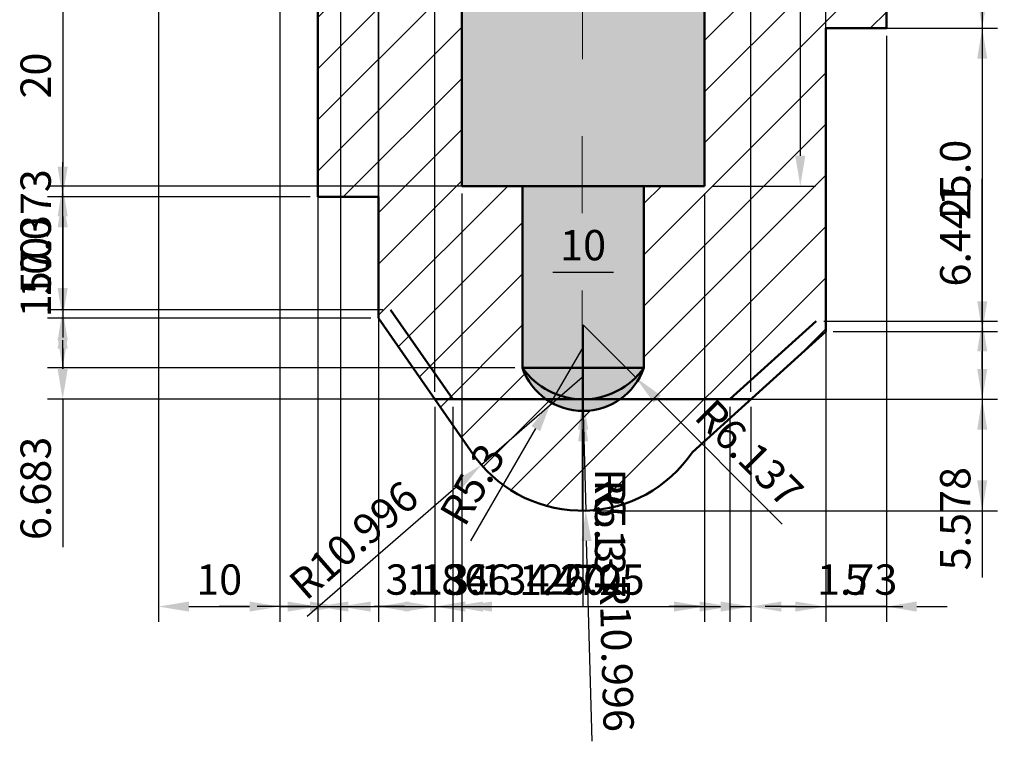
# Model space of a CAD drawing. Units: millimetres. Extents: x 1159 to 1466, y 1237 to 1440.
# Tile 4 of 6: x 1378 to 1459, y 1237 to 1296. Entities that reach past the tile are written whole.
import ezdxf

# ---------------------------------------------------------------- set-up
doc = ezdxf.new("R2010")
doc.units = ezdxf.units.MM
doc.linetypes.add('CENTER', pattern=[50.8, 31.75, -6.35, 6.35, -6.35])
for name, color, linetype, lineweight in [('M-CNTR', 1, 'CENTER', 18), ('M-DIMS', 2, 'Continuous', 25), ('M-HATC', 8, 'Continuous', 18), ('M-OUTL', 7, 'Continuous', 50)]:
    doc.layers.add(name, color=color, linetype=linetype, lineweight=lineweight)
doc.styles.get("Standard").update_dxf_attribs({"font": 'arial.ttf'})
doc.dimstyles.new('ISO-25', dxfattribs={"dimtxt": 2.5, "dimasz": 2.5, "dimexe": 1.25, "dimexo": 0.625, "dimtad": 1, "dimtxsty": 'Standard', "dimcen": 2.5, "dimadec": 0, "dimazin": 0, "dimtfac": 1, "dimtmove": 0, "dimatfit": 3, "dimfxl": 1, "dimarcsym": 0})

# ---------------------------------------------------------------- blocks, each defined once
blk = doc.blocks.new('*D42')
at = {"layer": 'Defpoints', "color": 0, "transparency": 16777216}
for p in [(1409.751, 1375.561), (1424.964, 1255.799), (1457.651, 1255.799)]:
    blk.add_point(p, dxfattribs=at)
at = {"layer": 'M-DIMS', "color": 0, "lineweight": -2, "transparency": 16777216}
for p, q in [((1410.376, 1375.561), (1458.901, 1375.561)), ((1457.651, 1373.061), (1457.651, 1258.299)), ((1425.589, 1255.799), (1458.901, 1255.799))]:
    blk.add_line(p, q, dxfattribs=at)
at = {"layer": 'M-DIMS', "color": 0, "transparency": 16777216}
for points in [[(1457.234, 1373.061), (1458.067, 1373.061), (1457.651, 1375.561)], [(1457.234, 1258.299), (1458.067, 1258.299), (1457.651, 1255.799)]]:
    blk.add_solid(points, dxfattribs=at)
at = {"layer": 'M-DIMS', "color": 0, "transparency": 16777216, "insert": (1455.749, 1315.68), "char_height": 2.5, "attachment_point": 5, "rotation": 90}
blk.add_mtext('119.76', dxfattribs=at)
blk = doc.blocks.new('*D44')
at = {"layer": 'Defpoints', "color": 0, "transparency": 16777216}
for p in [(1389.751, 1320.561), (1399.751, 1320.561), (1399.751, 1247.895)]:
    blk.add_point(p, dxfattribs=at)
at = {"layer": 'M-DIMS', "color": 0, "lineweight": -2, "transparency": 16777216}
for p, q in [((1389.751, 1319.936), (1389.751, 1246.645)), ((1399.751, 1319.936), (1399.751, 1246.645)), ((1392.251, 1247.895), (1397.251, 1247.895))]:
    blk.add_line(p, q, dxfattribs=at)
at = {"layer": 'M-DIMS', "color": 0, "transparency": 16777216}
for points in [[(1392.251, 1248.311), (1392.251, 1247.478), (1389.751, 1247.895)], [(1397.251, 1248.311), (1397.251, 1247.478), (1399.751, 1247.895)]]:
    blk.add_solid(points, dxfattribs=at)
at = {"layer": 'M-DIMS', "color": 0, "transparency": 16777216, "insert": (1394.751, 1249.796), "char_height": 2.5, "attachment_point": 5}
blk.add_mtext('10', dxfattribs=at)
blk = doc.blocks.new('*D46')
at = {"layer": 'Defpoints', "color": 0, "transparency": 16777216}
for p in [(1414.751, 1282.561), (1434.751, 1282.561), (1434.751, 1247.895)]:
    blk.add_point(p, dxfattribs=at)
at = {"layer": 'M-DIMS', "color": 0, "lineweight": -2, "transparency": 16777216}
for p, q in [((1414.751, 1281.936), (1414.751, 1246.645)), ((1434.751, 1281.936), (1434.751, 1246.645)), ((1417.251, 1247.895), (1432.251, 1247.895))]:
    blk.add_line(p, q, dxfattribs=at)
at = {"layer": 'M-DIMS', "color": 0, "transparency": 16777216}
for points in [[(1417.251, 1248.311), (1417.251, 1247.478), (1414.751, 1247.895)], [(1432.251, 1248.311), (1432.251, 1247.478), (1434.751, 1247.895)]]:
    blk.add_solid(points, dxfattribs=at)
at = {"layer": 'M-DIMS', "color": 0, "transparency": 16777216, "insert": (1424.751, 1249.796), "char_height": 2.5, "attachment_point": 5}
blk.add_mtext('20', dxfattribs=at)
blk = doc.blocks.new('*D47')
at = {"layer": 'Defpoints', "color": 0, "transparency": 16777216}
for p in [(1434.751, 1317.561), (1434.751, 1282.561), (1442.651, 1282.561)]:
    blk.add_point(p, dxfattribs=at)
at = {"layer": 'M-DIMS', "color": 0, "lineweight": -2, "transparency": 16777216}
for p, q in [((1435.376, 1317.561), (1443.901, 1317.561)), ((1442.651, 1315.061), (1442.651, 1285.061)), ((1435.376, 1282.561), (1443.901, 1282.561))]:
    blk.add_line(p, q, dxfattribs=at)
at = {"layer": 'M-DIMS', "color": 0, "transparency": 16777216}
for points in [[(1442.234, 1315.061), (1443.067, 1315.061), (1442.651, 1317.561)], [(1442.234, 1285.061), (1443.067, 1285.061), (1442.651, 1282.561)]]:
    blk.add_solid(points, dxfattribs=at)
at = {"layer": 'M-DIMS', "color": 0, "transparency": 16777216, "insert": (1440.749, 1300.061), "char_height": 2.5, "attachment_point": 5, "rotation": 90}
blk.add_mtext('35', dxfattribs=at)
blk = doc.blocks.new('*D48')
at = {"layer": 'Defpoints', "color": 0, "transparency": 16777216}
for p in [(1429.751, 1275.461), (1419.751, 1267.561), (1429.751, 1267.561)]:
    blk.add_point(p, dxfattribs=at)
at = {"layer": 'M-DIMS', "color": 0, "lineweight": -2, "transparency": 16777216}
for p, q in [((1419.751, 1268.186), (1419.751, 1276.711)), ((1429.751, 1268.186), (1429.751, 1276.711)), ((1422.251, 1275.461), (1427.251, 1275.461))]:
    blk.add_line(p, q, dxfattribs=at)
at = {"layer": 'M-DIMS', "color": 0, "transparency": 16777216}
for points in [[(1422.251, 1275.878), (1422.251, 1275.044), (1419.751, 1275.461)], [(1427.251, 1275.878), (1427.251, 1275.044), (1429.751, 1275.461)]]:
    blk.add_solid(points, dxfattribs=at)
at = {"layer": 'M-DIMS', "color": 0, "transparency": 16777216, "insert": (1424.751, 1277.362), "char_height": 2.5, "attachment_point": 5}
blk.add_mtext('10', dxfattribs=at)
blk = doc.blocks.new('*D49')
at = {"layer": 'Defpoints', "color": 0, "transparency": 16777216}
for p in [(1444.751, 1295.561), (1449.751, 1295.561), (1444.751, 1247.895)]:
    blk.add_point(p, dxfattribs=at)
at = {"layer": 'M-DIMS', "color": 0, "lineweight": -2, "transparency": 16777216}
for p, q in [((1444.751, 1294.936), (1444.751, 1246.645)), ((1449.751, 1294.936), (1449.751, 1246.645)), ((1442.251, 1247.895), (1439.751, 1247.895)), ((1449.751, 1247.895), (1444.751, 1247.895)), ((1452.251, 1247.895), (1454.751, 1247.895))]:
    blk.add_line(p, q, dxfattribs=at)
at = {"layer": 'M-DIMS', "color": 0, "transparency": 16777216}
for points in [[(1442.251, 1248.311), (1442.251, 1247.478), (1444.751, 1247.895)], [(1452.251, 1248.311), (1452.251, 1247.478), (1449.751, 1247.895)]]:
    blk.add_solid(points, dxfattribs=at)
at = {"layer": 'M-DIMS', "color": 0, "transparency": 16777216, "insert": (1447.251, 1249.791), "char_height": 2.5, "attachment_point": 5}
blk.add_mtext('5', dxfattribs=at)
blk = doc.blocks.new('*D50')
at = {"layer": 'Defpoints', "color": 0, "transparency": 16777216}
for p in [(1449.751, 1315.561), (1449.751, 1295.561), (1457.651, 1295.561)]:
    blk.add_point(p, dxfattribs=at)
at = {"layer": 'M-DIMS', "color": 0, "lineweight": -2, "transparency": 16777216}
for p, q in [((1450.376, 1315.561), (1458.901, 1315.561)), ((1457.651, 1313.061), (1457.651, 1298.061)), ((1450.376, 1295.561), (1458.901, 1295.561))]:
    blk.add_line(p, q, dxfattribs=at)
at = {"layer": 'M-DIMS', "color": 0, "transparency": 16777216}
for points in [[(1457.234, 1313.061), (1458.067, 1313.061), (1457.651, 1315.561)], [(1457.234, 1298.061), (1458.067, 1298.061), (1457.651, 1295.561)]]:
    blk.add_solid(points, dxfattribs=at)
at = {"layer": 'M-DIMS', "color": 0, "transparency": 16777216, "insert": (1455.749, 1305.561), "char_height": 2.5, "attachment_point": 5, "rotation": 90}
blk.add_mtext('20', dxfattribs=at)
blk = doc.blocks.new('*D51')
at = {"layer": 'Defpoints', "color": 0, "transparency": 16777216}
for p in [(1402.885, 1301.665), (1381.851, 1281.665), (1402.885, 1281.665)]:
    blk.add_point(p, dxfattribs=at)
at = {"layer": 'M-DIMS', "color": 0, "lineweight": -2, "transparency": 16777216}
for p, q in [((1402.26, 1301.665), (1380.601, 1301.665)), ((1381.851, 1299.165), (1381.851, 1284.165)), ((1402.26, 1281.665), (1380.601, 1281.665))]:
    blk.add_line(p, q, dxfattribs=at)
at = {"layer": 'M-DIMS', "color": 0, "transparency": 16777216}
for points in [[(1381.434, 1299.165), (1382.267, 1299.165), (1381.851, 1301.665)], [(1381.434, 1284.165), (1382.267, 1284.165), (1381.851, 1281.665)]]:
    blk.add_solid(points, dxfattribs=at)
at = {"layer": 'M-DIMS', "color": 0, "transparency": 16777216, "insert": (1379.949, 1291.665), "char_height": 2.5, "attachment_point": 5, "rotation": 90}
blk.add_mtext('20', dxfattribs=at)
blk = doc.blocks.new('*D54')
at = {"layer": 'Defpoints', "color": 0, "transparency": 16777216}
for p in [(1424.659, 1266.79), (1424.964, 1255.799)]:
    blk.add_point(p, dxfattribs=at)
at = {"layer": 'M-DIMS', "color": 0, "lineweight": -2, "transparency": 16777216}
for p, q in [((1424.659, 1266.79), (1424.964, 1255.799)), ((1425.492, 1236.787), (1425.033, 1253.3))]:
    blk.add_line(p, q, dxfattribs=at)
at = {"layer": 'M-DIMS', "color": 0, "transparency": 16777216}
blk.add_solid([(1425.45, 1253.311), (1424.617, 1253.288), (1424.964, 1255.799)], dxfattribs=at)
at = {"layer": 'M-DIMS', "color": 0, "transparency": 16777216, "insert": (1427.198, 1243.846), "char_height": 2.5, "attachment_point": 5, "rotation": 271.59062}
blk.add_mtext('R10.996', dxfattribs=at)
blk = doc.blocks.new('*D55')
at = {"layer": 'Defpoints', "color": 0, "transparency": 16777216}
for p in [(1424.751, 1271.12), (1424.751, 1264.983)]:
    blk.add_point(p, dxfattribs=at)
at = {"layer": 'M-DIMS', "color": 0, "lineweight": -2, "transparency": 16777216}
for p, q in [((1424.751, 1271.12), (1424.751, 1264.983)), ((1424.752, 1247.904), (1424.751, 1262.483))]:
    blk.add_line(p, q, dxfattribs=at)
at = {"layer": 'M-DIMS', "color": 0, "transparency": 16777216}
blk.add_solid([(1425.168, 1262.483), (1424.334, 1262.483), (1424.751, 1264.983)], dxfattribs=at)
at = {"layer": 'M-DIMS', "color": 0, "transparency": 16777216, "insert": (1426.654, 1253.943), "char_height": 2.5, "attachment_point": 5, "rotation": 270.0019}
blk.add_mtext('R6.137', dxfattribs=at)
blk = doc.blocks.new('*D56')
at = {"layer": 'Defpoints', "color": 0, "transparency": 16777216}
for p in [(1424.751, 1269.318), (1424.751, 1264.018)]:
    blk.add_point(p, dxfattribs=at)
at = {"layer": 'M-DIMS', "color": 0, "lineweight": -2, "transparency": 16777216}
for p, q in [((1424.751, 1269.318), (1424.751, 1264.018)), ((1424.752, 1250.824), (1424.751, 1261.518))]:
    blk.add_line(p, q, dxfattribs=at)
at = {"layer": 'M-DIMS', "color": 0, "transparency": 16777216}
blk.add_solid([(1425.168, 1261.518), (1424.334, 1261.518), (1424.751, 1264.018)], dxfattribs=at)
at = {"layer": 'M-DIMS', "color": 0, "transparency": 16777216, "insert": (1426.654, 1254.921), "char_height": 2.5, "attachment_point": 5, "rotation": 270.00221}
blk.add_mtext('R5.3', dxfattribs=at)
blk = doc.blocks.new('*D61')
at = {"layer": 'Defpoints', "color": 0, "transparency": 16777216}
for p in [(1444.751, 1295.561), (1444.751, 1270.561), (1457.651, 1270.561)]:
    blk.add_point(p, dxfattribs=at)
at = {"layer": 'M-DIMS', "color": 0, "lineweight": -2, "transparency": 16777216}
for p, q in [((1445.376, 1295.561), (1458.901, 1295.561)), ((1457.651, 1293.061), (1457.651, 1273.061)), ((1445.376, 1270.561), (1458.901, 1270.561))]:
    blk.add_line(p, q, dxfattribs=at)
at = {"layer": 'M-DIMS', "color": 0, "transparency": 16777216}
for points in [[(1457.234, 1293.061), (1458.067, 1293.061), (1457.651, 1295.561)], [(1457.234, 1273.061), (1458.067, 1273.061), (1457.651, 1270.561)]]:
    blk.add_solid(points, dxfattribs=at)
at = {"layer": 'M-DIMS', "color": 0, "transparency": 16777216, "insert": (1455.749, 1283.061), "char_height": 2.5, "attachment_point": 5, "rotation": 90}
blk.add_mtext('25.0', dxfattribs=at)
blk = doc.blocks.new('*D65')
at = {"layer": 'Defpoints', "color": 0, "transparency": 16777216}
for p in [(1399.751, 1315.561), (1402.885, 1301.665), (1402.885, 1247.895)]:
    blk.add_point(p, dxfattribs=at)
at = {"layer": 'M-DIMS', "color": 0, "lineweight": -2, "transparency": 16777216}
for p, q in [((1399.751, 1314.936), (1399.751, 1246.645)), ((1402.885, 1301.04), (1402.885, 1246.645)), ((1397.251, 1247.895), (1394.751, 1247.895)), ((1399.751, 1247.895), (1402.885, 1247.895)), ((1405.385, 1247.895), (1417.559, 1247.895))]:
    blk.add_line(p, q, dxfattribs=at)
at = {"layer": 'M-DIMS', "color": 0, "transparency": 16777216}
for points in [[(1397.251, 1248.311), (1397.251, 1247.478), (1399.751, 1247.895)], [(1405.385, 1248.311), (1405.385, 1247.478), (1402.885, 1247.895)]]:
    blk.add_solid(points, dxfattribs=at)
at = {"layer": 'M-DIMS', "color": 0, "transparency": 16777216, "insert": (1412.722, 1249.797), "char_height": 2.5, "attachment_point": 5}
blk.add_mtext('3.134', dxfattribs=at)
blk = doc.blocks.new('*D66')
at = {"layer": 'Defpoints', "color": 0, "transparency": 16777216}
for p in [(1404.751, 1315.561), (1402.885, 1301.665), (1404.751, 1247.895)]:
    blk.add_point(p, dxfattribs=at)
at = {"layer": 'M-DIMS', "color": 0, "lineweight": -2, "transparency": 16777216}
for p, q in [((1404.751, 1314.936), (1404.751, 1246.645)), ((1402.885, 1301.04), (1402.885, 1246.645)), ((1400.385, 1247.895), (1397.885, 1247.895)), ((1402.885, 1247.895), (1404.751, 1247.895)), ((1407.251, 1247.895), (1419.2, 1247.895))]:
    blk.add_line(p, q, dxfattribs=at)
at = {"layer": 'M-DIMS', "color": 0, "transparency": 16777216}
for points in [[(1400.385, 1248.311), (1400.385, 1247.478), (1402.885, 1247.895)], [(1407.251, 1248.311), (1407.251, 1247.478), (1404.751, 1247.895)]]:
    blk.add_solid(points, dxfattribs=at)
at = {"layer": 'M-DIMS', "color": 0, "transparency": 16777216, "insert": (1414.475, 1249.796), "char_height": 2.5, "attachment_point": 5}
blk.add_mtext('1.866', dxfattribs=at)
blk = doc.blocks.new('*D67')
at = {"layer": 'Defpoints', "color": 0, "transparency": 16777216}
for p in [(1404.751, 1315.561), (1407.885, 1311.665), (1407.885, 1247.895)]:
    blk.add_point(p, dxfattribs=at)
at = {"layer": 'M-DIMS', "color": 0, "lineweight": -2, "transparency": 16777216}
for p, q in [((1404.751, 1314.936), (1404.751, 1246.645)), ((1407.885, 1311.04), (1407.885, 1246.645)), ((1402.251, 1247.895), (1399.751, 1247.895)), ((1404.751, 1247.895), (1407.885, 1247.895)), ((1410.385, 1247.895), (1422.559, 1247.895))]:
    blk.add_line(p, q, dxfattribs=at)
at = {"layer": 'M-DIMS', "color": 0, "transparency": 16777216}
for points in [[(1402.251, 1248.311), (1402.251, 1247.478), (1404.751, 1247.895)], [(1410.385, 1248.311), (1410.385, 1247.478), (1407.885, 1247.895)]]:
    blk.add_solid(points, dxfattribs=at)
at = {"layer": 'M-DIMS', "color": 0, "transparency": 16777216, "insert": (1417.722, 1249.797), "char_height": 2.5, "attachment_point": 5}
blk.add_mtext('3.134', dxfattribs=at)
blk = doc.blocks.new('*D68')
at = {"layer": 'Defpoints', "color": 0, "transparency": 16777216}
for p in [(1402.885, 1281.665), (1381.851, 1271.665), (1407.885, 1271.665)]:
    blk.add_point(p, dxfattribs=at)
at = {"layer": 'M-DIMS', "color": 0, "lineweight": -2, "transparency": 16777216}
for p, q in [((1402.26, 1281.665), (1380.601, 1281.665)), ((1381.851, 1279.165), (1381.851, 1274.165)), ((1407.26, 1271.665), (1380.601, 1271.665))]:
    blk.add_line(p, q, dxfattribs=at)
at = {"layer": 'M-DIMS', "color": 0, "transparency": 16777216}
for points in [[(1381.434, 1279.165), (1382.267, 1279.165), (1381.851, 1281.665)], [(1381.434, 1274.165), (1382.267, 1274.165), (1381.851, 1271.665)]]:
    blk.add_solid(points, dxfattribs=at)
at = {"layer": 'M-DIMS', "color": 0, "transparency": 16777216, "insert": (1379.949, 1276.665), "char_height": 2.5, "attachment_point": 5, "rotation": 90}
blk.add_mtext('10.0', dxfattribs=at)
blk = doc.blocks.new('*D69')
at = {"layer": 'Defpoints', "color": 0, "transparency": 16777216}
for p in [(1407.885, 1271.665), (1381.851, 1264.983), (1412.534, 1264.983)]:
    blk.add_point(p, dxfattribs=at)
at = {"layer": 'M-DIMS', "color": 0, "lineweight": -2, "transparency": 16777216}
for p, q in [((1407.26, 1271.665), (1380.601, 1271.665)), ((1381.851, 1269.165), (1381.851, 1267.483)), ((1411.909, 1264.983), (1380.601, 1264.983)), ((1381.851, 1264.983), (1381.851, 1252.783))]:
    blk.add_line(p, q, dxfattribs=at)
at = {"layer": 'M-DIMS', "color": 0, "transparency": 16777216}
for points in [[(1381.434, 1269.165), (1382.267, 1269.165), (1381.851, 1271.665)], [(1381.434, 1267.483), (1382.267, 1267.483), (1381.851, 1264.983)]]:
    blk.add_solid(points, dxfattribs=at)
at = {"layer": 'M-DIMS', "color": 0, "transparency": 16777216, "insert": (1379.949, 1257.633), "char_height": 2.5, "attachment_point": 5, "rotation": 90}
blk.add_mtext('6.683', dxfattribs=at)
blk = doc.blocks.new('*D70')
at = {"layer": 'Defpoints', "color": 0, "transparency": 16777216}
for p in [(1444.751, 1270.561), (1438.586, 1264.983), (1457.651, 1264.983)]:
    blk.add_point(p, dxfattribs=at)
at = {"layer": 'M-DIMS', "color": 0, "lineweight": -2, "transparency": 16777216}
for p, q in [((1457.651, 1273.061), (1457.651, 1275.561)), ((1445.376, 1270.561), (1458.901, 1270.561)), ((1457.651, 1270.561), (1457.651, 1264.983)), ((1439.211, 1264.983), (1458.901, 1264.983)), ((1457.651, 1262.483), (1457.651, 1250.291))]:
    blk.add_line(p, q, dxfattribs=at)
at = {"layer": 'M-DIMS', "color": 0, "transparency": 16777216}
for points in [[(1457.234, 1273.061), (1458.067, 1273.061), (1457.651, 1270.561)], [(1457.234, 1262.483), (1458.067, 1262.483), (1457.651, 1264.983)]]:
    blk.add_solid(points, dxfattribs=at)
at = {"layer": 'M-DIMS', "color": 0, "transparency": 16777216, "insert": (1455.749, 1255.137), "char_height": 2.5, "attachment_point": 5, "rotation": 90}
blk.add_mtext('5.578', dxfattribs=at)
blk = doc.blocks.new('*D71')
at = {"layer": 'Defpoints', "color": 0, "transparency": 16777216}
for p in [(1443.97, 1271.424), (1457.651, 1271.424), (1436.851, 1264.983)]:
    blk.add_point(p, dxfattribs=at)
at = {"layer": 'M-DIMS', "color": 0, "lineweight": -2, "transparency": 16777216}
for p, q in [((1457.651, 1271.424), (1457.651, 1283.141)), ((1444.595, 1271.424), (1458.901, 1271.424)), ((1457.651, 1267.483), (1457.651, 1268.924)), ((1437.476, 1264.983), (1458.901, 1264.983))]:
    blk.add_line(p, q, dxfattribs=at)
at = {"layer": 'M-DIMS', "color": 0, "transparency": 16777216}
for points in [[(1457.234, 1268.924), (1458.067, 1268.924), (1457.651, 1271.424)], [(1457.234, 1267.483), (1458.067, 1267.483), (1457.651, 1264.983)]]:
    blk.add_solid(points, dxfattribs=at)
at = {"layer": 'M-DIMS', "color": 0, "transparency": 16777216, "insert": (1455.749, 1278.533), "char_height": 2.5, "attachment_point": 5, "rotation": 90}
blk.add_mtext('6.441', dxfattribs=at)
blk = doc.blocks.new('*D72')
at = {"layer": 'Defpoints', "color": 0, "transparency": 16777216}
for p in [(1381.851, 1272.355), (1408.877, 1272.355), (1414.006, 1264.983)]:
    blk.add_point(p, dxfattribs=at)
at = {"layer": 'M-DIMS', "color": 0, "lineweight": -2, "transparency": 16777216}
for p, q in [((1381.851, 1272.355), (1381.851, 1284.521)), ((1408.252, 1272.355), (1380.601, 1272.355)), ((1381.851, 1267.483), (1381.851, 1269.855)), ((1413.381, 1264.983), (1380.601, 1264.983))]:
    blk.add_line(p, q, dxfattribs=at)
at = {"layer": 'M-DIMS', "color": 0, "transparency": 16777216}
for points in [[(1381.434, 1269.855), (1382.267, 1269.855), (1381.851, 1272.355)], [(1381.434, 1267.483), (1382.267, 1267.483), (1381.851, 1264.983)]]:
    blk.add_solid(points, dxfattribs=at)
at = {"layer": 'M-DIMS', "color": 0, "transparency": 16777216, "insert": (1379.949, 1279.688), "char_height": 2.5, "attachment_point": 5, "rotation": 90}
blk.add_mtext('7.373', dxfattribs=at)
blk = doc.blocks.new('*D73')
at = {"layer": 'Defpoints', "color": 0, "transparency": 16777216}
for p in [(1412.534, 1264.983), (1438.586, 1264.983), (1438.586, 1247.895)]:
    blk.add_point(p, dxfattribs=at)
at = {"layer": 'M-DIMS', "color": 0, "lineweight": -2, "transparency": 16777216}
for p, q in [((1412.534, 1264.358), (1412.534, 1246.645)), ((1438.586, 1264.358), (1438.586, 1246.645)), ((1415.034, 1247.895), (1436.086, 1247.895))]:
    blk.add_line(p, q, dxfattribs=at)
at = {"layer": 'M-DIMS', "color": 0, "transparency": 16777216}
for points in [[(1415.034, 1248.311), (1415.034, 1247.478), (1412.534, 1247.895)], [(1436.086, 1248.311), (1436.086, 1247.478), (1438.586, 1247.895)]]:
    blk.add_solid(points, dxfattribs=at)
at = {"layer": 'M-DIMS', "color": 0, "transparency": 16777216, "insert": (1425.56, 1249.796), "char_height": 2.5, "attachment_point": 5}
blk.add_mtext('26.05', dxfattribs=at)
blk = doc.blocks.new('*D74')
at = {"layer": 'Defpoints', "color": 0, "transparency": 16777216}
for p in [(1412.534, 1383.461), (1407.885, 1271.665), (1412.534, 1264.983)]:
    blk.add_point(p, dxfattribs=at)
at = {"layer": 'M-DIMS', "color": 0, "lineweight": -2, "transparency": 16777216}
for p, q in [((1407.885, 1272.29), (1407.885, 1384.711)), ((1412.534, 1265.608), (1412.534, 1384.711)), ((1405.385, 1383.461), (1402.885, 1383.461)), ((1407.885, 1383.461), (1412.534, 1383.461)), ((1415.034, 1383.461), (1427.326, 1383.461))]:
    blk.add_line(p, q, dxfattribs=at)
at = {"layer": 'M-DIMS', "color": 0, "transparency": 16777216}
for points in [[(1405.385, 1383.878), (1405.385, 1383.044), (1407.885, 1383.461)], [(1415.034, 1383.878), (1415.034, 1383.044), (1412.534, 1383.461)]]:
    blk.add_solid(points, dxfattribs=at)
at = {"layer": 'M-DIMS', "color": 0, "transparency": 16777216, "insert": (1422.43, 1385.362), "char_height": 2.5, "attachment_point": 5}
blk.add_mtext('4.649', dxfattribs=at)
blk = doc.blocks.new('*D75')
at = {"layer": 'Defpoints', "color": 0, "transparency": 16777216}
for p in [(1444.751, 1383.461), (1444.751, 1270.561), (1438.586, 1264.983)]:
    blk.add_point(p, dxfattribs=at)
at = {"layer": 'M-DIMS', "color": 0, "lineweight": -2, "transparency": 16777216}
for p, q in [((1438.586, 1265.608), (1438.586, 1384.711)), ((1444.751, 1271.186), (1444.751, 1384.711)), ((1436.086, 1383.461), (1433.586, 1383.461)), ((1438.586, 1383.461), (1444.751, 1383.461)), ((1447.251, 1383.461), (1459.469, 1383.461))]:
    blk.add_line(p, q, dxfattribs=at)
at = {"layer": 'M-DIMS', "color": 0, "transparency": 16777216}
for points in [[(1436.086, 1383.878), (1436.086, 1383.044), (1438.586, 1383.461)], [(1447.251, 1383.878), (1447.251, 1383.044), (1444.751, 1383.461)]]:
    blk.add_solid(points, dxfattribs=at)
at = {"layer": 'M-DIMS', "color": 0, "transparency": 16777216, "insert": (1454.61, 1385.362), "char_height": 2.5, "attachment_point": 5}
blk.add_mtext('6.165', dxfattribs=at)
blk = doc.blocks.new('*D76')
at = {"layer": 'Defpoints', "color": 0, "transparency": 16777216}
for p in [(1412.534, 1264.983), (1414.006, 1264.983), (1414.006, 1247.895)]:
    blk.add_point(p, dxfattribs=at)
at = {"layer": 'M-DIMS', "color": 0, "lineweight": -2, "transparency": 16777216}
for p, q in [((1412.534, 1264.358), (1412.534, 1246.645)), ((1414.006, 1264.358), (1414.006, 1246.645)), ((1410.034, 1247.895), (1407.534, 1247.895)), ((1412.534, 1247.895), (1414.006, 1247.895)), ((1416.506, 1247.895), (1428.432, 1247.895))]:
    blk.add_line(p, q, dxfattribs=at)
at = {"layer": 'M-DIMS', "color": 0, "transparency": 16777216}
for points in [[(1410.034, 1248.311), (1410.034, 1247.478), (1412.534, 1247.895)], [(1416.506, 1248.311), (1416.506, 1247.478), (1414.006, 1247.895)]]:
    blk.add_solid(points, dxfattribs=at)
at = {"layer": 'M-DIMS', "color": 0, "transparency": 16777216, "insert": (1423.719, 1249.775), "char_height": 2.5, "attachment_point": 5}
blk.add_mtext('1.472', dxfattribs=at)
blk = doc.blocks.new('*D77')
at = {"layer": 'Defpoints', "color": 0, "transparency": 16777216}
for p in [(1436.851, 1264.983), (1438.586, 1264.983), (1438.586, 1247.895)]:
    blk.add_point(p, dxfattribs=at)
at = {"layer": 'M-DIMS', "color": 0, "lineweight": -2, "transparency": 16777216}
for p, q in [((1436.851, 1264.358), (1436.851, 1246.645)), ((1438.586, 1264.358), (1438.586, 1246.645)), ((1434.351, 1247.895), (1431.851, 1247.895)), ((1436.851, 1247.895), (1438.586, 1247.895)), ((1441.086, 1247.895), (1451.094, 1247.895))]:
    blk.add_line(p, q, dxfattribs=at)
at = {"layer": 'M-DIMS', "color": 0, "transparency": 16777216}
for points in [[(1434.351, 1248.311), (1434.351, 1247.478), (1436.851, 1247.895)], [(1441.086, 1248.311), (1441.086, 1247.478), (1438.586, 1247.895)]]:
    blk.add_solid(points, dxfattribs=at)
at = {"layer": 'M-DIMS', "color": 0, "transparency": 16777216, "insert": (1447.34, 1249.797), "char_height": 2.5, "attachment_point": 5}
blk.add_mtext('1.73', dxfattribs=at)
blk = doc.blocks.new('*D78')
at = {"layer": 'Defpoints', "color": 0, "transparency": 16777216}
for p in [(1419.751, 1282.561), (1381.851, 1267.561), (1419.751, 1267.561)]:
    blk.add_point(p, dxfattribs=at)
at = {"layer": 'M-DIMS', "color": 0, "lineweight": -2, "transparency": 16777216}
for p, q in [((1419.126, 1282.561), (1380.601, 1282.561)), ((1381.851, 1280.061), (1381.851, 1270.061)), ((1419.126, 1267.561), (1380.601, 1267.561))]:
    blk.add_line(p, q, dxfattribs=at)
at = {"layer": 'M-DIMS', "color": 0, "transparency": 16777216}
for points in [[(1381.434, 1280.061), (1382.267, 1280.061), (1381.851, 1282.561)], [(1381.434, 1270.061), (1382.267, 1270.061), (1381.851, 1267.561)]]:
    blk.add_solid(points, dxfattribs=at)
at = {"layer": 'M-DIMS', "color": 0, "transparency": 16777216, "insert": (1379.949, 1275.061), "char_height": 2.5, "attachment_point": 5, "rotation": 90}
blk.add_mtext('15.0', dxfattribs=at)
blk = doc.blocks.new('*D88')
at = {"layer": 'Defpoints', "color": 0, "transparency": 16777216}
for p in [(1424.659, 1266.79), (1416.362, 1259.575)]:
    blk.add_point(p, dxfattribs=at)
at = {"layer": 'M-DIMS', "color": 0, "lineweight": -2, "transparency": 16777216}
for p, q in [((1424.659, 1266.79), (1416.362, 1259.575)), ((1402.01, 1247.094), (1414.475, 1257.934))]:
    blk.add_line(p, q, dxfattribs=at)
at = {"layer": 'M-DIMS', "color": 0, "transparency": 16777216}
blk.add_solid([(1414.202, 1258.249), (1414.749, 1257.62), (1416.362, 1259.575)], dxfattribs=at)
at = {"layer": 'M-DIMS', "color": 0, "transparency": 16777216, "insert": (1406.052, 1253.129), "char_height": 2.5, "attachment_point": 5, "rotation": 41.01102}
blk.add_mtext('R10.996', dxfattribs=at)
blk = doc.blocks.new('*D89')
at = {"layer": 'Defpoints', "color": 0, "transparency": 16777216}
for p in [(1424.751, 1271.12), (1429.085, 1266.775)]:
    blk.add_point(p, dxfattribs=at)
at = {"layer": 'M-DIMS', "color": 0, "lineweight": -2, "transparency": 16777216}
for p, q in [((1424.751, 1271.12), (1429.085, 1266.775)), ((1441.147, 1254.683), (1430.851, 1265.005))]:
    blk.add_line(p, q, dxfattribs=at)
at = {"layer": 'M-DIMS', "color": 0, "transparency": 16777216}
blk.add_solid([(1431.146, 1265.299), (1430.556, 1264.711), (1429.085, 1266.775)], dxfattribs=at)
at = {"layer": 'M-DIMS', "color": 0, "transparency": 16777216, "insert": (1438.228, 1260.303), "char_height": 2.5, "attachment_point": 5, "rotation": 314.92911}
blk.add_mtext('R6.137', dxfattribs=at)
blk = doc.blocks.new('*D90')
at = {"layer": 'Defpoints', "color": 0, "transparency": 16777216}
for p in [(1424.751, 1269.318), (1422.1, 1264.729)]:
    blk.add_point(p, dxfattribs=at)
at = {"layer": 'M-DIMS', "color": 0, "lineweight": -2, "transparency": 16777216}
for p, q in [((1424.751, 1269.318), (1422.1, 1264.729)), ((1415.499, 1253.305), (1420.849, 1262.565))]:
    blk.add_line(p, q, dxfattribs=at)
at = {"layer": 'M-DIMS', "color": 0, "transparency": 16777216}
blk.add_solid([(1420.488, 1262.773), (1421.21, 1262.356), (1422.1, 1264.729)], dxfattribs=at)
at = {"layer": 'M-DIMS', "color": 0, "transparency": 16777216, "insert": (1415.902, 1257.804), "char_height": 2.5, "attachment_point": 5, "rotation": 59.98324}
blk.add_mtext('R5.3', dxfattribs=at)

msp = doc.modelspace()

# ---------------------------------------------------------------- hatches: boundary and pattern name
at = {"layer": 'M-HATC'}
h = msp.add_hatch(dxfattribs=at)
h.set_pattern_fill('ANSI31', color=256, scale=0.94)
h.set_pattern_definition([(45, (0, -76.8912), (-2.11036, 2.11036), [])])
h.paths.add_polyline_path([(1414.6374, 1375.561), (1409.7508, 1375.561), (1409.7508, 1335.561), (1414.6374, 1335.561)])
h.paths.add_polyline_path([(1439.7508, 1375.561), (1434.4515, 1375.561), (1434.4515, 1335.561), (1439.7508, 1335.561)])
h.paths.add_polyline_path([(1449.7508, 1315.561), (1444.7508, 1315.561), (1444.7508, 1320.561), (1449.7508, 1320.561), (1449.7508, 1335.561), (1439.7508, 1335.561), (1439.7508, 1320.561), (1429.7508, 1320.561), (1429.7508, 1317.561), (1434.7508, 1317.561), (1434.7508, 1282.561), (1429.7508, 1282.561), (1429.7508, 1267.561, -0.1562704), (1427.7989, 1264.9827), (1438.5857, 1264.9827), (1444.7508, 1270.561), (1444.7508, 1275.561), (1444.7508, 1295.561), (1449.7508, 1295.561)])
h.paths.add_polyline_path([(1414.7508, 1317.561), (1419.7508, 1317.561), (1419.7508, 1320.561), (1409.7508, 1320.561), (1409.7508, 1335.561), (1399.7508, 1335.561), (1399.7508, 1330.561), (1389.7508, 1330.561), (1389.7508, 1320.561), (1399.7508, 1320.561), (1399.7508, 1315.561), (1404.7508, 1315.561), (1407.8849, 1311.6652), (1407.8849, 1301.6652), (1402.8849, 1301.6652), (1402.8849, 1281.6652), (1407.8849, 1281.6652), (1407.8849, 1271.6652), (1412.5343, 1264.9827), (1421.7027, 1264.9827, -0.1562704), (1419.7508, 1267.561), (1419.7508, 1282.561), (1414.7508, 1282.561)])
h.paths.add_polyline_path([(1424.6651, 1264.0191, -0.1502665), (1421.7027, 1264.9827), (1412.5343, 1264.9827), (1415.9205, 1260.1158, 0.2337513), (1424.6588, 1255.7945)])
h.paths.add_polyline_path([(1433.7538, 1260.6108), (1438.5857, 1264.9827), (1427.7989, 1264.9827, -0.1585441), (1424.6651, 1264.0191), (1424.6588, 1255.7945, 0.248431)])
h = msp.add_hatch(color=256, dxfattribs=at)
h.set_gradient(color1=(34, 52, 110), color2=(0, 0, 0))
h.paths.add_polyline_path([(1424.7508, 1375.561), (1414.6374, 1375.561), (1414.6374, 1335.561), (1424.7201, 1335.561)])
h.paths.add_polyline_path([(1434.4515, 1375.561), (1424.7508, 1375.561), (1424.7201, 1335.561), (1434.4515, 1335.561)])
h.paths.add_polyline_path([(1424.7201, 1335.561), (1414.6374, 1335.561), (1409.7508, 1335.561), (1409.7508, 1320.561), (1424.7085, 1320.561)])
h.paths.add_polyline_path([(1439.7508, 1335.561), (1424.7201, 1335.561), (1424.7085, 1320.561), (1424.7508, 1320.561), (1439.7508, 1320.561)])
h.paths.add_polyline_path([(1434.7508, 1317.561), (1429.7508, 1317.561), (1424.7062, 1317.561), (1424.6793, 1282.561), (1424.7508, 1282.561), (1434.7508, 1282.561)])
h.paths.add_polyline_path([(1424.7062, 1317.561), (1419.7508, 1317.561), (1414.7508, 1317.561), (1414.7508, 1282.561), (1424.6793, 1282.561)])
h.paths.add_polyline_path([(1424.6793, 1282.561), (1419.7508, 1282.561), (1419.7508, 1267.561), (1424.6678, 1267.561)])
h.paths.add_polyline_path([(1429.7508, 1282.561), (1424.6793, 1282.561), (1424.6678, 1267.561), (1429.7508, 1267.561)])
h.paths.add_polyline_path([(1424.6678, 1267.561), (1419.7508, 1267.561, 0.2389901), (1424.6658, 1264.9833)])
h.paths.add_polyline_path([(1429.7508, 1267.561), (1424.6678, 1267.561), (1424.6658, 1264.9833, 0.2463189)])
h.paths.add_polyline_path([(1419.7508, 1267.561, 0.1562704), (1421.7027, 1264.9827), (1424.7508, 1264.9827, -0.2426514)])
h.paths.add_polyline_path([(1429.7508, 1267.561, -0.2426514), (1424.7508, 1264.9827), (1427.7989, 1264.9827, 0.1562704)], flags=17)
h.paths.add_polyline_path([(1427.7989, 1264.9827), (1424.7508, 1264.9827), (1424.6658, 1264.9827), (1424.6651, 1264.0191, 0.1585441)])
h.paths.add_polyline_path([(1424.6658, 1264.9827), (1421.7027, 1264.9827, 0.1502665), (1424.6651, 1264.0191)])

# ---------------------------------------------------------------- linework, layer by layer
at = {"layer": 'M-CNTR'}
msp.add_line((1424.7508, 1375.561), (1424.6588, 1255.7945), dxfattribs=at)
at = {"layer": 'M-OUTL'}
for p, q in [((1414.7508, 1317.561), (1414.7508, 1282.561)), ((1434.7508, 1282.561), (1434.7508, 1317.561)), ((1449.7508, 1315.561), (1449.7508, 1295.561)), ((1402.8849, 1301.6652), (1402.8849, 1281.6652)), ((1449.7508, 1295.561), (1444.7508, 1295.561)), ((1444.7508, 1295.561), (1444.7508, 1275.561)), ((1414.7508, 1282.561), (1434.7508, 1282.561)), ((1424.7508, 1282.561), (1419.7508, 1282.561)), ((1419.7508, 1282.561), (1419.7508, 1267.561)), ((1429.7508, 1267.561), (1429.7508, 1282.561)), ((1402.8849, 1281.6652), (1407.8849, 1281.6652)), ((1407.8849, 1281.6652), (1407.8849, 1271.6652)), ((1444.7508, 1275.561), (1444.7508, 1270.561)), ((1408.8767, 1272.3552), (1414.0062, 1264.9827)), ((1407.8849, 1271.6652), (1415.9205, 1260.1158)), ((1443.9699, 1271.4241), (1436.8508, 1264.9827)), ((1444.7508, 1270.561), (1433.7538, 1260.6108)), ((1419.7508, 1267.561), (1429.7508, 1267.561)), ((1424.7508, 1264.9827), (1412.5343, 1264.9827)), ((1424.7508, 1264.9827), (1438.5857, 1264.9827))]:
    msp.add_line(p, q, dxfattribs=at)
for centre, radius, start, end in [((1424.7508, 1271.12), 6.1373, 215.442848, 324.557152), ((1424.7508, 1269.3182), 5.2998, 199.363556, 340.636444), ((1424.6588, 1266.7903), 10.9957, 217.373074, 325.806418)]:
    msp.add_arc(centre, radius, start, end, dxfattribs=at)

# ---------------------------------------------------------------- dimensions: what is measured, and where the dimension line sits
at = {"layer": 'M-DIMS'}
for base, p1, p2, override, picture, middle in [((1412.5343, 1383.461), (1407.8849, 1271.6652), (1412.5343, 1264.9827), {"dimdec": 3, "dimlfac": 1, "dimrnd": 0, "dimzin": 0, "dimdsep": 46, "dimlunit": 2}, '*D74', (1422.4303, 1385.3624)), ((1444.7508, 1383.461), (1438.5857, 1264.9827), (1444.7508, 1270.561), {"dimdec": 3, "dimlfac": 1, "dimrnd": 0, "dimzin": 0, "dimdsep": 46, "dimlunit": 2}, '*D75', (1454.6101, 1385.3624)), ((1399.7508, 1247.8945), (1389.7508, 1320.561), (1399.7508, 1320.561), {"dimdec": 0, "dimlfac": 1, "dimrnd": 0, "dimzin": 0, "dimdsep": 46, "dimlunit": 2}, '*D44', (1394.7508, 1249.796)), ((1402.8849, 1247.8945), (1399.7508, 1315.561), (1402.8849, 1301.6652), {"dimdec": 3, "dimlfac": 1, "dimrnd": 0, "dimzin": 0, "dimdsep": 46, "dimlunit": 2}, '*D65', (1412.722, 1249.7968)), ((1404.7508, 1247.8945), (1402.8849, 1301.6652), (1404.7508, 1315.561), {"dimdec": 3, "dimlfac": 1, "dimrnd": 0, "dimzin": 0, "dimdsep": 46, "dimlunit": 2}, '*D66', (1414.4754, 1249.796)), ((1407.8849, 1247.8945), (1404.7508, 1315.561), (1407.8849, 1311.6652), {"dimdec": 3, "dimlfac": 1, "dimrnd": 0, "dimzin": 0, "dimdsep": 46, "dimlunit": 2}, '*D67', (1417.722, 1249.7968)), ((1444.7508, 1247.8945), (1449.7508, 1295.561), (1444.7508, 1295.561), {"dimdec": 0, "dimlfac": 1, "dimrnd": 0, "dimzin": 0, "dimdsep": 46, "dimlunit": 2}, '*D49', (1447.2508, 1249.7909)), ((1434.7508, 1247.8945), (1414.7508, 1282.561), (1434.7508, 1282.561), {"dimdec": 0, "dimlfac": 1, "dimrnd": 0, "dimzin": 0, "dimdsep": 46, "dimlunit": 2}, '*D46', (1424.7508, 1249.796)), ((1429.7508, 1275.461), (1419.7508, 1267.561), (1429.7508, 1267.561), {"dimdec": 0, "dimlfac": 1, "dimrnd": 0, "dimzin": 0, "dimdsep": 46, "dimlunit": 2}, '*D48', (1424.7508, 1277.3624)), ((1414.0062, 1247.8945), (1412.5343, 1264.9827), (1414.0062, 1264.9827), {"dimdec": 3, "dimlfac": 1, "dimrnd": 0, "dimzin": 0, "dimdsep": 46, "dimlunit": 2}, '*D76', (1423.7189, 1249.7747)), ((1438.5857, 1247.8945), (1412.5343, 1264.9827), (1438.5857, 1264.9827), {"dimdec": 2, "dimlfac": 1, "dimrnd": 0, "dimzin": 0, "dimdsep": 46, "dimlunit": 2}, '*D73', (1425.56, 1249.796)), ((1438.5857, 1247.8945), (1436.8508, 1264.9827), (1438.5857, 1264.9827), {"dimdec": 2, "dimlfac": 1, "dimrnd": 0, "dimzin": 0, "dimdsep": 46, "dimlunit": 2}, '*D77', (1447.3399, 1249.7968))]:
    dim = msp.add_linear_dim(base=base, p1=p1, p2=p2, dimstyle='ISO-25', override=override, dxfattribs=at)
    dim.commit()
    dim.dimension.update_dxf_attribs({"geometry": picture, "text_midpoint": middle})
for base, p1, p2, angle, override, picture, middle in [((1457.6508, 1255.7988), (1409.7508, 1375.561), (1424.9638, 1255.7988), 90, {"dimdec": 2, "dimlfac": 1, "dimrnd": 0, "dimzin": 0, "dimdsep": 46, "dimlunit": 2}, '*D42', (1455.7494, 1315.6799)), ((1442.6508, 1282.561), (1434.7508, 1317.561), (1434.7508, 1282.561), 270, {"dimdec": 0, "dimlfac": 1, "dimrnd": 0, "dimzin": 0, "dimdsep": 46, "dimlunit": 2}, '*D47', (1440.7485, 1300.061)), ((1457.6508, 1295.561), (1449.7508, 1315.561), (1449.7508, 1295.561), 270, {"dimdec": 0, "dimlfac": 1, "dimrnd": 0, "dimzin": 0, "dimdsep": 46, "dimlunit": 2}, '*D50', (1455.7494, 1305.561)), ((1381.8508, 1281.6652), (1402.8849, 1301.6652), (1402.8849, 1281.6652), 90, {"dimdec": 0, "dimlfac": 1, "dimrnd": 0, "dimzin": 0, "dimdsep": 46, "dimlunit": 2}, '*D51', (1379.9494, 1291.6652)), ((1457.6508, 1270.561), (1444.7508, 1295.561), (1444.7508, 1270.561), 90, {"dimdec": 1, "dimlfac": 1, "dimrnd": 0, "dimzin": 0, "dimdsep": 46, "dimlunit": 2}, '*D61', (1455.7494, 1283.061)), ((1381.8508, 1272.35524), (1414.00622, 1264.98268), (1408.87669, 1272.35524), 90, {"dimdec": 3, "dimlfac": 1, "dimrnd": 0, "dimzin": 0, "dimdsep": 46, "dimlunit": 2}, '*D72', (1379.94851, 1279.68812)), ((1381.8508, 1267.561), (1419.7508, 1282.561), (1419.7508, 1267.561), 90, {"dimdec": 1, "dimlfac": 1, "dimrnd": 0, "dimzin": 0, "dimdsep": 46, "dimlunit": 2}, '*D78', (1379.9494, 1275.061)), ((1457.6508, 1271.4241), (1436.8508, 1264.9827), (1443.9699, 1271.4241), 90, {"dimdec": 3, "dimlfac": 1, "dimrnd": 0, "dimzin": 0, "dimdsep": 46, "dimlunit": 2}, '*D71', (1455.7494, 1278.5327)), ((1381.8508, 1271.6652), (1402.8849, 1281.6652), (1407.8849, 1271.6652), 90, {"dimdec": 1, "dimlfac": 1, "dimrnd": 0, "dimzin": 0, "dimdsep": 46, "dimlunit": 2}, '*D68', (1379.9494, 1276.6652)), ((1457.6508, 1264.9827), (1444.7508, 1270.561), (1438.5857, 1264.9827), 90, {"dimdec": 3, "dimlfac": 1, "dimrnd": 0, "dimzin": 0, "dimdsep": 46, "dimlunit": 2}, '*D70', (1455.7494, 1255.137)), ((1381.8508, 1264.98268), (1407.88489, 1271.66519), (1412.53431, 1264.98268), 90, {"dimdec": 3, "dimlfac": 1, "dimrnd": 0, "dimzin": 0, "dimdsep": 46, "dimlunit": 2}, '*D69', (1379.94851, 1257.63275))]:
    dim = msp.add_linear_dim(base=base, p1=p1, p2=p2, angle=angle, dimstyle='ISO-25', override=override, dxfattribs=at)
    dim.commit()
    dim.dimension.update_dxf_attribs({"geometry": picture, "text_midpoint": middle})
for center, mpoint, override, picture, middle in [((1424.7508, 1271.12), (1424.751, 1264.9827), {"dimdec": 3, "dimlfac": 1, "dimrnd": 0, "dimzin": 0, "dimdsep": 46, "dimlunit": 2}, '*D55', (1426.6537, 1253.9434)), ((1424.7508, 1271.12), (1429.0851, 1266.7749), {"dimdec": 3, "dimlfac": 1, "dimrnd": 0, "dimzin": 0, "dimdsep": 46, "dimlunit": 2}, '*D89', (1438.2283, 1260.3027)), ((1424.7508, 1269.3182), (1422.0996, 1264.7292), {"dimdec": 1, "dimlfac": 1, "dimrnd": 0, "dimzin": 0, "dimdsep": 46, "dimlunit": 2}, '*D90', (1415.9016, 1257.8039)), ((1424.7508, 1269.3182), (1424.751, 1264.0184), {"dimdec": 1, "dimlfac": 1, "dimrnd": 0, "dimzin": 0, "dimdsep": 46, "dimlunit": 2}, '*D56', (1426.6536, 1254.9215)), ((1424.6588, 1266.7903), (1416.3616, 1259.5748), {"dimdec": 3, "dimlfac": 1, "dimrnd": 0, "dimzin": 0, "dimdsep": 46, "dimlunit": 2}, '*D88', (1406.0515, 1253.1288)), ((1424.6588, 1266.7903), (1424.964, 1255.7988), {"dimdec": 3, "dimlfac": 1, "dimrnd": 0, "dimzin": 0, "dimdsep": 46, "dimlunit": 2}, '*D54', (1427.1981, 1243.8465))]:
    dim = msp.add_radius_dim(center=center, mpoint=mpoint, dimstyle='ISO-25', override=override, dxfattribs=at)
    dim.commit()
    dim.dimension.update_dxf_attribs({"geometry": picture, "text_midpoint": middle})

doc.saveas('drawing.dxf')
